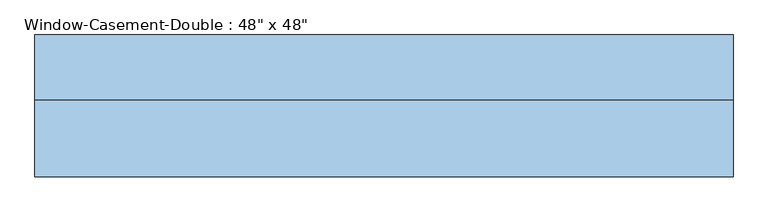
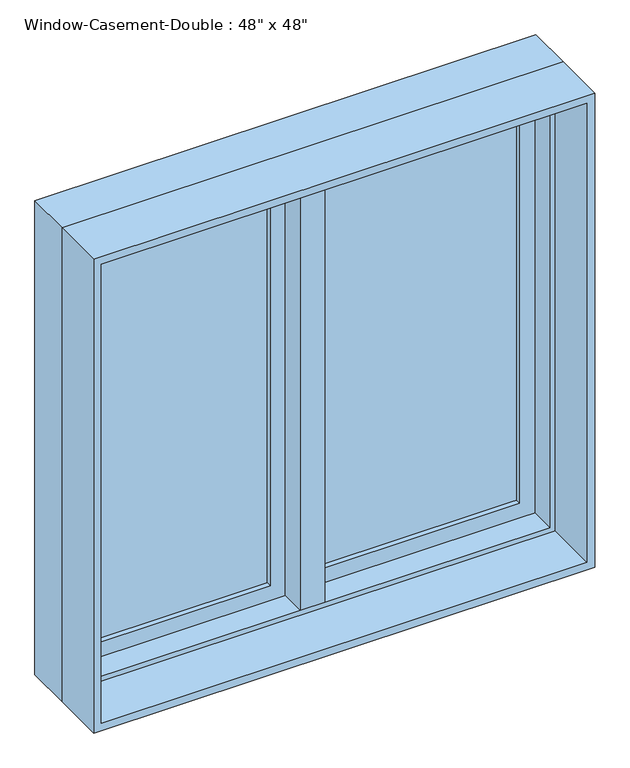
"""IFC4 building model written with IfcOpenShell, lengths in millimetres: window geometry."""

from ifc_helpers import new_model, si_unit, frame, origin, place, context, project, spatial, polyline, outline, extrude, faceted_brep, source, transform, mapped, element, save


def window_af3140d2(model_context):
    return source(origin(), model_context, "Body", "SolidModel", [
        faceted_brep([(9.525, 133.35, 2120.9), (-9.525, 133.35, 2120.9), (-9.525, 82.55, 2120.9), (9.525, 82.55, 2120.9), (9.525, 133.35, 927.1), (9.525, 82.55, 927.1), (-9.525, 82.55, 927.1), (-9.525, 133.35, 927.1), (-9.525, 82.55, 946.15), (-9.525, 82.55, 2101.85), (-30.1625, 82.55, 946.15), (-30.1625, 82.55, 2101.85), (-30.1625, 19.05, 946.15), (-30.1625, 19.05, 2101.85), (30.1625, 19.05, 946.15), (30.1625, 19.05, 2101.85), (30.1625, 82.55, 946.15), (30.1625, 82.55, 2101.85), (9.525, 82.55, 946.15), (9.525, 82.55, 2101.85)], [[[0, 1, 2, 3]], [[4, 5, 6, 7]], [[1, 0, 4, 7]], [[2, 1, 7, 6, 8, 9]], [[9, 8, 10, 11]], [[11, 10, 12, 13]], [[13, 12, 14, 15]], [[15, 14, 16, 17]], [[17, 16, 18, 19]], [[0, 3, 19, 18, 5, 4]], [[18, 8, 6, 5]], [[9, 19, 3, 2]], [[8, 18, 16, 14, 12, 10]], [[19, 9, 11, 13, 15, 17]]]),
        extrude(outline(polyline([(-66.675, 114.3), (-66.675, 107.95), (-539.75, 107.95), (-539.75, 114.3), (-66.675, 114.3)])), frame((0.0, 0.0, 984.25), z_axis=(0.0, 0.0, 1.0), x_axis=(1.0, 0.0, 0.0)), (0.0, 0.0, 1.0), 1079.5),
        extrude(outline(polyline([(-539.75, 95.25), (-539.75, 101.6), (-66.675, 101.6), (-66.675, 95.25), (-539.75, 95.25)])), frame((0.0, 0.0, 984.25), z_axis=(0.0, 0.0, 1.0), x_axis=(1.0, 0.0, 0.0)), (0.0, 0.0, 1.0), 1079.5),
        extrude(outline(polyline([(539.75, 114.3), (539.75, 107.95), (66.675, 107.95), (66.675, 114.3), (539.75, 114.3)])), frame((0.0, 0.0, 984.25), z_axis=(0.0, 0.0, 1.0), x_axis=(1.0, 0.0, 0.0)), (0.0, 0.0, 1.0), 1079.5),
        extrude(outline(polyline([(66.675, 95.25), (66.675, 101.6), (539.75, 101.6), (539.75, 95.25), (66.675, 95.25)])), frame((0.0, 0.0, 984.25), z_axis=(0.0, 0.0, 1.0), x_axis=(1.0, 0.0, 0.0)), (0.0, 0.0, 1.0), 1079.5),
        extrude(outline(polyline([(2120.9, -596.9), (927.1, -596.9), (927.1, -9.525), (2120.9, -9.525), (2120.9, -596.9)]), holes=[polyline([(2063.75, -66.675), (984.25, -66.675), (984.25, -539.75), (2063.75, -539.75), (2063.75, -66.675)])]), frame((0.0, 82.55, 0.0), z_axis=(0.0, 1.0, 0.0), x_axis=(0.0, 0.0, 1.0)), (0.0, 0.0, 1.0), 44.45),
        extrude(outline(polyline([(927.1, 596.9), (2120.9, 596.9), (2120.9, 9.525), (927.1, 9.525), (927.1, 596.9)]), holes=[polyline([(984.25, 66.675), (2063.75, 66.675), (2063.75, 539.75), (984.25, 539.75), (984.25, 66.675)])]), frame((0.0, 82.55, 0.0), z_axis=(0.0, 1.0, 0.0), x_axis=(0.0, 0.0, 1.0)), (0.0, 0.0, 1.0), 44.45),
        extrude(outline(polyline([(2133.6, -609.6), (914.4, -609.6), (914.4, 609.6), (2133.6, 609.6), (2133.6, -609.6)]), holes=[polyline([(2114.55, 590.55), (933.45, 590.55), (933.45, -590.55), (2114.55, -590.55), (2114.55, 590.55)])]), frame((0.0, -114.3, 0.0), z_axis=(0.0, 1.0, 0.0), x_axis=(0.0, 0.0, 1.0)), (0.0, 0.0, 1.0), 133.35),
        faceted_brep([(577.85, 82.55, 2101.85), (577.85, 19.05, 2101.85), (-577.85, 19.05, 2101.85), (-577.85, 82.55, 2101.85), (596.9, 133.35, 2120.9), (596.9, 82.55, 2120.9), (-596.9, 82.55, 2120.9), (-596.9, 133.35, 2120.9), (609.6, 19.05, 2133.6), (609.6, 133.35, 2133.6), (-609.6, 133.35, 2133.6), (-609.6, 19.05, 2133.6), (-577.85, 19.05, 946.15), (-577.85, 82.55, 946.15), (-596.9, 82.55, 927.1), (-596.9, 133.35, 927.1), (-609.6, 133.35, 914.4), (-609.6, 19.05, 914.4), (577.85, 19.05, 946.15), (577.85, 82.55, 946.15), (596.9, 82.55, 927.1), (596.9, 133.35, 927.1), (609.6, 133.35, 914.4), (609.6, 19.05, 914.4)], [[[0, 1, 2, 3]], [[4, 5, 6, 7]], [[8, 9, 10, 11]], [[3, 2, 12, 13]], [[7, 6, 14, 15]], [[11, 10, 16, 17]], [[13, 12, 18, 19]], [[15, 14, 20, 21]], [[17, 16, 22, 23]], [[11, 17, 23, 8], [1, 18, 12, 2]], [[19, 18, 1, 0]], [[5, 20, 14, 6], [3, 13, 19, 0]], [[21, 20, 5, 4]], [[23, 22, 9, 8]], [[9, 22, 16, 10], [7, 15, 21, 4]]]),
    ])


if __name__ == "__main__":
    model = new_model("IFC4")
    model_context = context("Model", 3, world=origin())
    ifc_project = project(units=[si_unit("LENGTHUNIT", "METRE", prefix="MILLI")], contexts=[model_context])
    site = spatial("IfcSite", under=ifc_project)
    building = spatial("IfcBuilding", under=site)
    placement = place(None, origin())
    window_shape = window_af3140d2(model_context)
    element("IfcWindow", 1, ObjectType="Window-Casement-Double : 48\" x 48\"", at=placement, inside=building, context=model_context, shape_type="MappedRepresentation", body=[
        mapped(window_shape, transform((0.0, 0.0, 0.0), x_axis=(1.0, 0.0, 0.0), y_axis=(0.0, 1.0, 0.0), z_axis=(0.0, 0.0, 1.0))),
    ])
    save(model, "model.ifc")

# Revit data of these elements
# Type "Window-Casement-Double : 48\" x 48\""
#   Type Mark = "W"
#   Fire Rating = "0.5h"
#   Assembly Code = "B2020100"
#   Analytic Construction = "Double glazing - domestic"
#   Frame Extension [instance default] = 0' - 0 1/4"
#   Window Inset [instance default] = 0' - 0"
#   Wall Thickness [instance default] = 0' - 6"
#   Interior Wall Closure [instance default] = 0' - 2 1/4"
#   Half Width = 2' - 0"
#   Visual Light Transmittance = 0.81
#   Thermal Resistance (R) = 1.8146 (h·ft²·°F)/BTU
#   Solar Heat Gain Coefficient = 0.76
#   Rough Width = 4' - 0 1/2"
#   Rough Height = 4' - 0 1/2"
#   Height = 4' - 0"
#   Heat Transfer Coefficient (U) = 0.5511 BTU/(h·ft²·°F)
#   Exterior Wall Closure [instance default] = 0' - 1 1/4"
#   Extension Jamb [instance default] = 0' - 2 1/4"
#   Default Sill Height = 3' - 0"
#   Width = 4' - 0"
#   Define Thermal Properties by = 0
#   Muntin Visibility = yes
#   Interior Trim Visibility [instance default] = yes
#   Exterior Trim Visibility [instance default] = yes
#   Extension Jamb Visibility [instance default] = yes
#   Interior Trim Material = Wood - Stained
#   Muntin Pattern = Muntin Pattern_2x2 : Muntin Pattern_2x2
#   Interior Trim = Trim-Window-Interior-Flat : Picture Frame
#   Interior Frame Material = Wood - Stained
#   Glass Panel Material = Glass
#   Exterior Trim Material = Clad - White
#   Exterior Trim = Trim-Window-Exterior-Flat : with Sill
#   Exterior Frame Material = Clad - White
#   Wall Closure = (empty or 0)
# Element 1 (IfcWindow, "Window-Casement-Double : 48\" x 48\"")
#   Wall Thickness = 0' - 9"
#   Extension Jamb = 0' - 5 1/4"
#   Materials on its faces: "Wood - Stained", "Glass", "Clad - White"
# Materials
#   "Wood - Stained": class "Wood", colour RGB 224 178 126, transparency 0, Cost = 0
#   "Glass": class "Glass", colour RGB 0 128 192, transparency 0.75, Description = "Soda Lime Glass", Cost = 0
#   "Clad - White": class "Wood", colour RGB 242 242 238, transparency 0, Cost = 0
